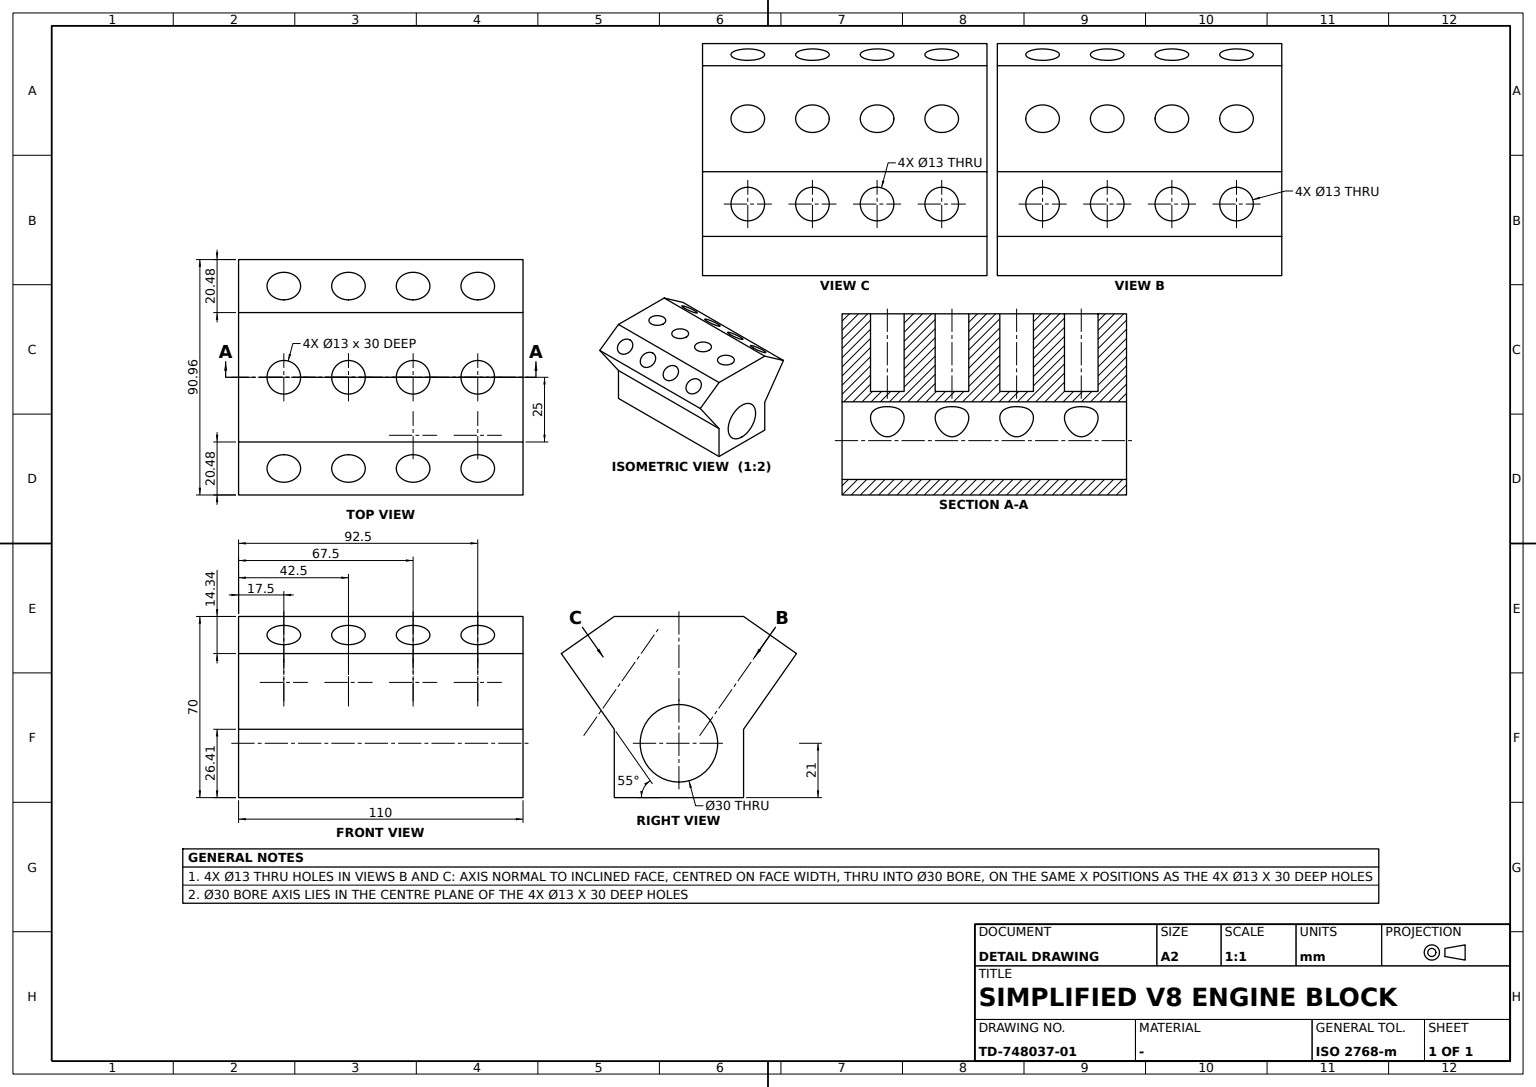
CATIA V5 part; units mm, degrees
sketch "Sketch1" plane through (0, 0, 0) normal (1, 0, 0) x (0, 1, 0)
  line L0 (25, 0) -> (25, 26.41)
  point P0 (45.48, 0)
  circle A0 centre (0, 21) radius 15
  point P1 (0, 21)
  line L1 (25, 26.41) -> (45.48, 55.6585)
  line L2 (45.48, 55.6585) -> (25, 69.9987)
  point P2 (25, 69.9987)
  point P3 (-45.48, 0)
  line L3 (-25, 0) -> (-25, 26.41)
  line L4 (-25, 26.41) -> (-45.48, 55.6585)
  line L5 (-45.48, 55.6585) -> (-25, 69.9987)
  line L6 (-25, 69.9987) -> (25, 69.9987)
  line L7 (-25, 0) -> (25, 0)
  dimension "length L0" = 26.41
  dimension "radius A0" = 15
  dimension "distance P1 origin" = 21
  dimension "distance origin P0" = 45.48
  constraint vertical L0 y-axis
  constraint coincidence P2 L0
  constraint horizontal L6 x-axis
  constraint horizontal L7 x-axis
extrude "Pad1" add sketch "Sketch1" along normal blind 110
sketch "Sketch2" plane through (0, 0, 69.9987) normal (0, 0, 1) x (1, 0, 0)
  circle A0 centre (17.5, 0) radius 6.5
  point P0 (17.5, 0)
  circle A1 centre (42.5, 0) radius 6.5
  point P1 (42.5, 0)
  circle A2 centre (67.5, 0) radius 6.5
  point P2 (67.5, 0)
  circle A3 centre (92.5, 0) radius 6.5
  point P3 (92.5, 0)
  dimension "radius A0" = 6.5
  dimension "distance P0 y axis" = 17.5
  dimension "radius A1" = 6.5
  dimension "distance P1 y axis" = 42.5
  dimension "radius A2" = 6.5
  dimension "distance P2 y axis" = 67.5
  dimension "radius A3" = 6.5
  dimension "distance P3 y axis" = 92.5
  constraint coincidence P0 x-axis
  constraint coincidence P1 x-axis
  constraint coincidence P2 x-axis
  constraint coincidence P3 x-axis
extrude "Pocket1" cut sketch "Sketch2" against normal blind 30
sketch "Sketch3" plane through (0, 41.1134, 58.716) normal (0, 0.5736, 0.8192) x (-1, 0, 0)
  circle A0 centre (-92.5, 7.1708) radius 6.5
  circle A1 centre (-67.5, 7.1708) radius 6.5
  circle A2 centre (-42.5, 7.1708) radius 6.5
  circle A3 centre (-17.5, 7.1708) radius 6.5
  point P0 (-17.5, 7.1708)
  dimension "radius A0" = 6.5
  dimension "radius A1" = 6.5
  dimension "radius A2" = 6.5
  dimension "distance P0 y axis" = 17.5
extrude "Pocket2" cut sketch "Sketch3" against normal up to next
mirror "Mirror1" about plane through (0, 0, 0) normal (0, 1, 0) of "Pocket2"
